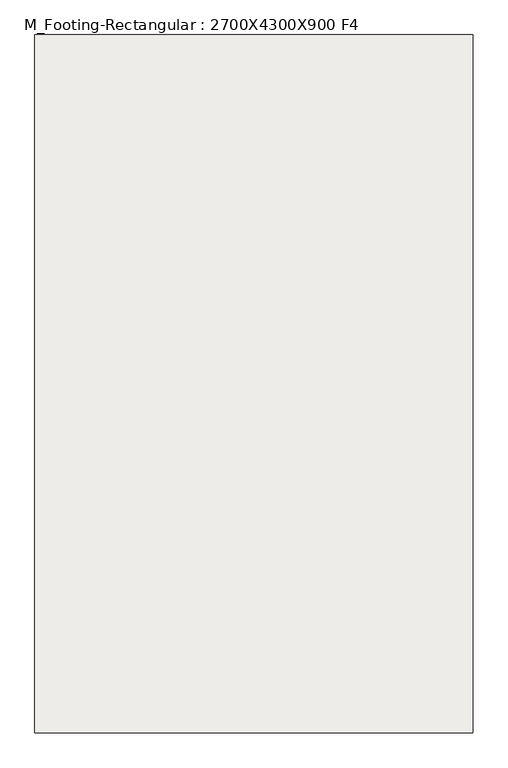
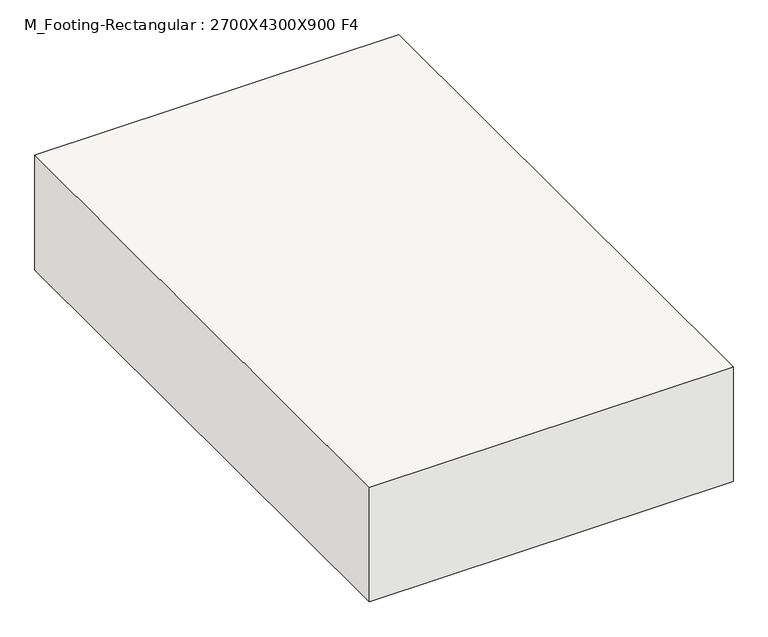
"""IFC4 building model written with IfcOpenShell, lengths in millimetres: slab geometry, M_Footing-Rectangular : 2700X4300X900 F4."""

from ifc_helpers import new_model, si_unit, frame, origin, place, context, project, spatial, polyline, outline, extrude, source, transform, mapped, element, save


def m_footing_rectangular_2700x4300x900_f4_c3563192(model_context):
    return source(origin(), model_context, "Body", "SweptSolid", [
        extrude(outline(polyline([(1350.0, 2150.0), (1350.0, -2150.0), (-1350.0, -2150.0), (-1350.0, 2150.0), (1350.0, 2150.0)])), frame((0.0, 0.0, -900.0), z_axis=(0.0, 0.0, 1.0), x_axis=(1.0, 0.0, 0.0)), (0.0, 0.0, 1.0), 900.0),
    ])


if __name__ == "__main__":
    model = new_model("IFC4")
    model_context = context("Model", 3, world=origin())
    ifc_project = project(units=[si_unit("LENGTHUNIT", "METRE", prefix="MILLI")], contexts=[model_context])
    site = spatial("IfcSite", under=ifc_project)
    building = spatial("IfcBuilding", under=site)
    placement = place(None, origin())
    m_footing_rectangular_2700x4300x900_f4_shape = m_footing_rectangular_2700x4300x900_f4_c3563192(model_context)
    element("IfcSlab", 1, ObjectType="M_Footing-Rectangular : 2700X4300X900 F4", at=placement, inside=building, context=model_context, shape_type="MappedRepresentation", body=[
        mapped(m_footing_rectangular_2700x4300x900_f4_shape, transform((0.0, 0.0, 0.0), x_axis=(1.0, 0.0, 0.0), y_axis=(0.0, 1.0, 0.0), z_axis=(0.0, 0.0, 1.0))),
    ])
    save(model, "model.ifc")

# Revit data of these elements
# Type "M_Footing-Rectangular : 2700X4300X900 F4"
#   Width = 2700 mm
#   Length = 4300 mm
#   Foundation Thickness = 900 mm
#   Structural Material [instance default] = Concrete, Cast-in-Place gray
#   Assembly Code = ""
# Element 1 (IfcSlab, "M_Footing-Rectangular : 2700X4300X900 F4")
#   Structural Material = Concrete, Cast In Situ
#   Materials on its faces: "Concrete, Cast In Situ"
# Materials
#   "Concrete, Cast-in-Place gray": class "Concrete", colour RGB 192 192 192, transparency 0, Description = "Cast-in-place concrete", Cost = 0
#   "Concrete, Cast In Situ": class "Concrete", colour RGB 192 192 192, transparency 0, Description = "physical material", Cost = 0
